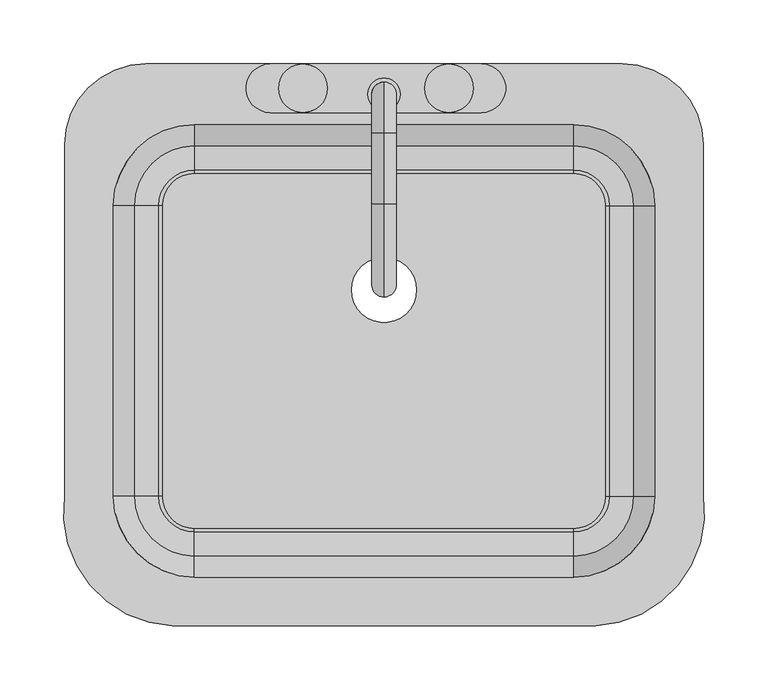
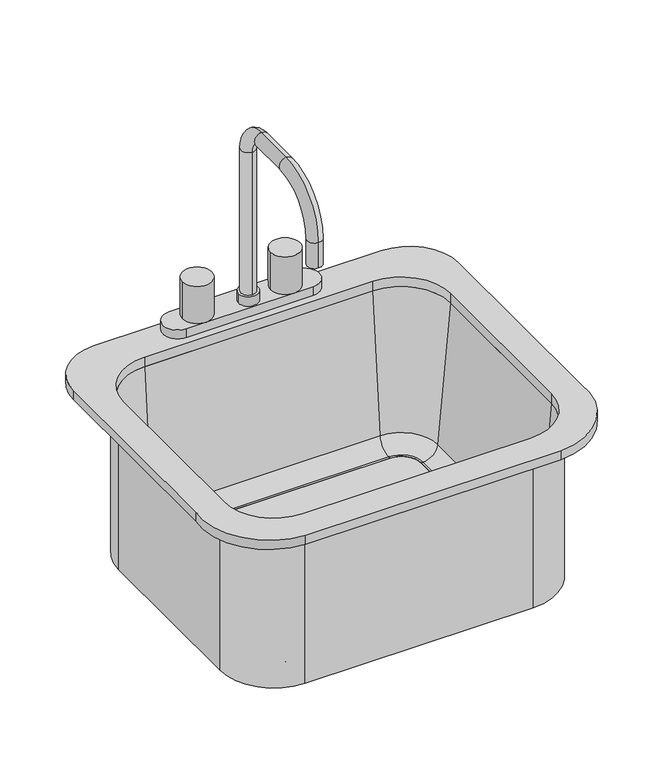
"""IFC4 building model written with IfcOpenShell, lengths in millimetres: flow terminal geometry."""

from ifc_helpers import new_model, si_unit, point, frame, frame_2d, origin, place, context, project, spatial, polyline, circle_curve, ellipse_curve, trimmed, segment, composite_curve, outline, extrude, source, transform, mapped, element, save
from ifc_brep_helpers import plane_surface, cylinder_surface, revolved_surface, advanced_brep


def flow_terminal_f629513f(model_context):
    return source(origin(), model_context, "Body", "SolidModel", [
        extrude(outline(composite_curve([segment(trimmed(circle_curve(frame_2d((-146.1534746, -170.8793432)), 89.0566732), [point((-149.9606923, -259.8545989))], [point((-234.3107593, -158.2545982))], False, "CARTESIAN"), True, "CONTINUOUS"), segment(polyline([(-234.3107593, -158.2545982), (-234.3107593, 116.6454011)]), True, "CONTINUOUS"), segment(trimmed(circle_curve(frame_2d((-170.8107593, 116.6454011)), 63.5), [point((-234.3107593, 116.6454011))], [point((-170.8107593, 180.1454011))], False, "CARTESIAN"), True, "CONTINUOUS"), segment(polyline([(-170.8107593, 180.1454011), (202.1892406, 180.1454011)]), True, "CONTINUOUS"), segment(trimmed(circle_curve(frame_2d((202.1892406, 116.6454011)), 63.5), [point((202.1892406, 180.1454011))], [point((265.6892406, 116.6454011))], False, "CARTESIAN"), True, "CONTINUOUS"), segment(polyline([(265.6892406, 116.6454011), (265.6892406, -158.2545989)]), True, "CONTINUOUS"), segment(trimmed(circle_curve(frame_2d((177.5319557, -170.8793432)), 89.0566732), [point((265.6892406, -158.2545989))], [point((181.3391735, -259.8545989))], False, "CARTESIAN"), True, "CONTINUOUS"), segment(polyline([(181.3391735, -259.8545989), (-149.9606923, -259.8545989)]), True, "CONTINUOUS")], self_intersect=False), holes=[composite_curve([segment(polyline([(164.0892406, 132.5204011), (-132.7107594, 132.5204011)]), True, "CONTINUOUS"), segment(trimmed(circle_curve(frame_2d((-132.7107594, 69.0204011)), 63.5), [point((-132.7107594, 132.5204011))], [point((-196.2107594, 69.0204011))], True, "CARTESIAN"), True, "CONTINUOUS"), segment(polyline([(-196.2107594, 69.0204011), (-196.2107594, -158.2545989)]), True, "CONTINUOUS"), segment(trimmed(circle_curve(frame_2d((-132.7107594, -158.2545989)), 63.5), [point((-196.2107594, -158.2545989))], [point((-132.7107594, -221.7545989))], True, "CARTESIAN"), True, "CONTINUOUS"), segment(polyline([(-132.7107594, -221.7545989), (164.0892406, -221.7545989)]), True, "CONTINUOUS"), segment(trimmed(circle_curve(frame_2d((164.0892406, -158.2545989)), 63.5), [point((164.0892406, -221.7545989))], [point((227.5892406, -158.2545989))], True, "CARTESIAN"), True, "CONTINUOUS"), segment(polyline([(227.5892406, -158.2545989), (227.5892406, 69.0204011)]), True, "CONTINUOUS"), segment(trimmed(circle_curve(frame_2d((164.0892406, 69.0204011)), 63.5), [point((227.5892406, 69.0204011))], [point((164.0892406, 132.5204011))], True, "CARTESIAN"), True, "CONTINUOUS")], self_intersect=False)]), frame((0.0, 0.0, 750.0), z_axis=(0.0, 0.0, 1.0), x_axis=(1.0, 0.0, 0.0)), (0.0, 0.0, 1.0), 12.7),
        advanced_brep(
        [(233.9392406, 69.0204011, 534.1), (164.0892406, 138.8704011, 534.1), (164.0892406, 138.8704011, 750.0), (233.9392406, 69.0204011, 750.0), (189.4892406, 69.0204011, 534.1), (164.0892406, 94.4204011, 534.1), (189.4892406, 69.0204011, 543.625), (164.0892406, 94.4204011, 543.625), (192.0776588, 69.0204011, 543.625), (164.0892406, 97.0088193, 543.625), (211.0551678, 69.0204011, 561.0146831), (164.0892406, 115.9863283, 561.0146831), (227.5892406, 69.0204011, 750.0), (164.0892406, 132.5204011, 750.0), (233.9392406, -158.2545989, 750.0), (233.9392406, -158.2545989, 534.1), (189.4892406, -158.2545989, 534.1), (189.4892406, -158.2545989, 543.625), (192.0776588, -158.2545989, 543.625), (211.0551678, -158.2545989, 561.0146831), (227.5892406, -158.2545989, 750.0), (164.0892406, -228.1045989, 534.1), (164.0892406, -228.1045989, 750.0), (164.0892406, -183.6545989, 534.1), (164.0892406, -183.6545989, 543.625), (164.0892406, -186.2430171, 543.625), (164.0892406, -205.2205261, 561.0146831), (164.0892406, -221.7545989, 750.0), (-132.7107594, -228.1045989, 750.0), (-132.7107594, -228.1045989, 534.1), (-132.7107594, -183.6545989, 534.1), (-132.7107594, -183.6545989, 543.625), (-132.7107594, -186.2430171, 543.625), (-132.7107594, -205.2205261, 561.0146831), (-132.7107594, -221.7545989, 750.0), (-202.5607594, -158.2545989, 534.1), (-202.5607594, -158.2545989, 750.0), (-158.1107594, -158.2545989, 534.1), (-158.1107594, -158.2545989, 543.625), (-160.6991776, -158.2545989, 543.625), (-179.6766866, -158.2545989, 561.0146831), (-196.2107594, -158.2545989, 750.0), (-202.5607594, 69.0204011, 750.0), (-202.5607594, 69.0204011, 534.1), (-158.1107594, 69.0204011, 534.1), (-158.1107594, 69.0204011, 543.625), (-160.6991776, 69.0204011, 543.625), (-179.6766866, 69.0204011, 561.0146831), (-196.2107594, 69.0204011, 750.0), (-132.7107594, 138.8704011, 534.1), (-132.7107594, 138.8704011, 750.0), (-132.7107594, 94.4204011, 534.1), (-132.7107594, 94.4204011, 543.625), (-132.7107594, 97.0088193, 543.625), (-132.7107594, 115.9863283, 561.0146831), (-132.7107594, 132.5204011, 750.0)],
        [
            (0, 1, circle_curve(frame((164.0892406, 69.0204011, 534.1), z_axis=(0.0, 0.0, 1.0), x_axis=(0.0, 1.0, 0.0)), 69.85)),
            (1, 2),
            (2, 3, circle_curve(frame((164.0892406, 69.0204011, 750.0), z_axis=(0.0, 0.0, -1.0), x_axis=(0.0, 1.0, 0.0)), 69.85)),
            (3, 0),
            (4, 5, circle_curve(frame((164.0892406, 69.0204011, 534.1), z_axis=(0.0, 0.0, 1.0), x_axis=(0.0, 1.0, 0.0)), 25.4)),
            (5, 1),
            (0, 4),
            (6, 7, circle_curve(frame((164.0892406, 69.0204011, 543.625), z_axis=(0.0, 0.0, 1.0), x_axis=(0.0, 1.0, 0.0)), 25.4)),
            (7, 5),
            (4, 6),
            (8, 9, circle_curve(frame((164.0892406, 69.0204011, 543.625), z_axis=(0.0, 0.0, 1.0), x_axis=(0.0, 1.0, 0.0)), 27.9884182)),
            (9, 7),
            (6, 8),
            (10, 11, circle_curve(frame((164.0892406, 69.0204011, 561.0146831), z_axis=(0.0, 0.0, 1.0), x_axis=(0.0, 1.0, 0.0)), 46.9659272)),
            (11, 9, circle_curve(frame((164.0892406, 97.0088193, 562.675), z_axis=(-1.0, 0.0, 0.0), x_axis=(0.0, 1.0, 0.0)), 19.05)),
            (8, 10, circle_curve(frame((192.0776588, 69.0204011, 562.675), z_axis=(0.0, -1.0, 0.0), x_axis=(1.0, 0.0, 0.0)), 19.05)),
            (12, 13, circle_curve(frame((164.0892406, 69.0204011, 750.0), z_axis=(0.0, 0.0, 1.0), x_axis=(0.0, 1.0, 0.0)), 63.5)),
            (13, 11),
            (10, 12),
            (2, 13),
            (12, 3),
            (3, 14),
            (14, 15),
            (15, 0),
            (15, 16),
            (16, 4),
            (16, 17),
            (17, 6),
            (17, 18),
            (18, 8),
            (18, 19, circle_curve(frame((192.0776588, -158.2545989, 562.675), z_axis=(0.0, -1.0, 0.0), x_axis=(1.0, 0.0, 0.0)), 19.05)),
            (19, 10),
            (19, 20),
            (20, 12),
            (20, 14),
            (21, 15, circle_curve(frame((164.0892406, -158.2545989, 534.1), z_axis=(0.0, 0.0, 1.0), x_axis=(1.0, 0.0, 0.0)), 69.85)),
            (14, 22, circle_curve(frame((164.0892406, -158.2545989, 750.0), z_axis=(0.0, 0.0, -1.0), x_axis=(1.0, 0.0, 0.0)), 69.85)),
            (22, 21),
            (23, 16, circle_curve(frame((164.0892406, -158.2545989, 534.1), z_axis=(0.0, 0.0, 1.0), x_axis=(1.0, 0.0, 0.0)), 25.4)),
            (21, 23),
            (24, 17, circle_curve(frame((164.0892406, -158.2545989, 543.625), z_axis=(0.0, 0.0, 1.0), x_axis=(1.0, 0.0, 0.0)), 25.4)),
            (23, 24),
            (25, 18, circle_curve(frame((164.0892406, -158.2545989, 543.625), z_axis=(0.0, 0.0, 1.0), x_axis=(1.0, 0.0, 0.0)), 27.9884182)),
            (24, 25),
            (26, 19, circle_curve(frame((164.0892406, -158.2545989, 561.0146831), z_axis=(0.0, 0.0, 1.0), x_axis=(1.0, 0.0, 0.0)), 46.9659272)),
            (25, 26, circle_curve(frame((164.0892406, -186.2430171, 562.675), z_axis=(-1.0, 0.0, 0.0), x_axis=(0.0, -1.0, 0.0)), 19.05)),
            (27, 20, circle_curve(frame((164.0892406, -158.2545989, 750.0), z_axis=(0.0, 0.0, 1.0), x_axis=(1.0, 0.0, 0.0)), 63.5)),
            (26, 27),
            (27, 22),
            (22, 28),
            (28, 29),
            (29, 21),
            (29, 30),
            (30, 23),
            (30, 31),
            (31, 24),
            (31, 32),
            (32, 25),
            (32, 33, circle_curve(frame((-132.7107594, -186.2430171, 562.675), z_axis=(-1.0, 0.0, 0.0), x_axis=(0.0, -1.0, 0.0)), 19.05)),
            (33, 26),
            (33, 34),
            (34, 27),
            (34, 28),
            (35, 29, circle_curve(frame((-132.7107594, -158.2545989, 534.1), z_axis=(0.0, 0.0, 1.0), x_axis=(0.0, -1.0, 0.0)), 69.85)),
            (28, 36, circle_curve(frame((-132.7107594, -158.2545989, 750.0), z_axis=(0.0, 0.0, -1.0), x_axis=(0.0, -1.0, 0.0)), 69.85)),
            (36, 35),
            (37, 30, circle_curve(frame((-132.7107594, -158.2545989, 534.1), z_axis=(0.0, 0.0, 1.0), x_axis=(0.0, -1.0, 0.0)), 25.4)),
            (35, 37),
            (38, 31, circle_curve(frame((-132.7107594, -158.2545989, 543.625), z_axis=(0.0, 0.0, 1.0), x_axis=(0.0, -1.0, 0.0)), 25.4)),
            (37, 38),
            (39, 32, circle_curve(frame((-132.7107594, -158.2545989, 543.625), z_axis=(0.0, 0.0, 1.0), x_axis=(0.0, -1.0, 0.0)), 27.9884182)),
            (38, 39),
            (40, 33, circle_curve(frame((-132.7107594, -158.2545989, 561.0146831), z_axis=(0.0, 0.0, 1.0), x_axis=(0.0, -1.0, 0.0)), 46.9659272)),
            (39, 40, circle_curve(frame((-160.6991776, -158.2545989, 562.675), z_axis=(0.0, 1.0, 0.0), x_axis=(-1.0, 0.0, 0.0)), 19.05)),
            (41, 34, circle_curve(frame((-132.7107594, -158.2545989, 750.0), z_axis=(0.0, 0.0, 1.0), x_axis=(0.0, -1.0, 0.0)), 63.5)),
            (40, 41),
            (41, 36),
            (36, 42),
            (42, 43),
            (43, 35),
            (43, 44),
            (44, 37),
            (44, 45),
            (45, 38),
            (45, 46),
            (46, 39),
            (46, 47, circle_curve(frame((-160.6991776, 69.0204011, 562.675), z_axis=(0.0, 1.0, 0.0), x_axis=(-1.0, 0.0, 0.0)), 19.05)),
            (47, 40),
            (47, 48),
            (48, 41),
            (48, 42),
            (49, 43, circle_curve(frame((-132.7107594, 69.0204011, 534.1), z_axis=(0.0, 0.0, 1.0), x_axis=(-1.0, 0.0, 0.0)), 69.85)),
            (42, 50, circle_curve(frame((-132.7107594, 69.0204011, 750.0), z_axis=(0.0, 0.0, -1.0), x_axis=(-1.0, 0.0, 0.0)), 69.85)),
            (50, 49),
            (51, 44, circle_curve(frame((-132.7107594, 69.0204011, 534.1), z_axis=(0.0, 0.0, 1.0), x_axis=(-1.0, 0.0, 0.0)), 25.4)),
            (49, 51),
            (52, 45, circle_curve(frame((-132.7107594, 69.0204011, 543.625), z_axis=(0.0, 0.0, 1.0), x_axis=(-1.0, 0.0, 0.0)), 25.4)),
            (51, 52),
            (53, 46, circle_curve(frame((-132.7107594, 69.0204011, 543.625), z_axis=(0.0, 0.0, 1.0), x_axis=(-1.0, 0.0, 0.0)), 27.9884182)),
            (52, 53),
            (54, 47, circle_curve(frame((-132.7107594, 69.0204011, 561.0146831), z_axis=(0.0, 0.0, 1.0), x_axis=(-1.0, 0.0, 0.0)), 46.9659272)),
            (53, 54, circle_curve(frame((-132.7107594, 97.0088193, 562.675), z_axis=(1.0, 0.0, 0.0), x_axis=(0.0, 1.0, 0.0)), 19.05)),
            (55, 48, circle_curve(frame((-132.7107594, 69.0204011, 750.0), z_axis=(0.0, 0.0, 1.0), x_axis=(-1.0, 0.0, 0.0)), 63.5)),
            (54, 55),
            (55, 50),
            (50, 2),
            (1, 49),
            (5, 51),
            (7, 52),
            (9, 53),
            (11, 54),
            (13, 55),
        ],
        [
            cylinder_surface(frame((164.0892406, 69.0204011, 0.0), z_axis=(0.0, 0.0, -1.0), x_axis=(0.0, 1.0, 0.0)), 69.85),
            plane_surface(frame((164.0892406, 69.0204011, 534.1), z_axis=(0.0, 0.0, -1.0), x_axis=(0.0, 1.0, 0.0))),
            revolved_surface(polyline([(164.0892406, 94.42040109999999, 534.1), (164.0892406, 94.42040109999999, 543.625)]), (164.0892406, 69.0204011, 0.0), (0.0, 0.0, -1.0)),
            plane_surface(frame((164.0892406, 69.0204011, 543.625), z_axis=(0.0, 0.0, 1.0), x_axis=(0.0, 1.0, 0.0))),
            revolved_surface(trimmed(ellipse_curve(frame((164.0892406, 97.0088193, 562.675), z_axis=(1.0, 0.0, 0.0), x_axis=(0.0, 1.0, 0.0)), 19.05, 19.05), [point((164.0892406, 97.0088193, 543.625))], [point((164.0892406, 115.9863283, 561.0146831))], True, "CARTESIAN"), (164.0892406, 69.0204011, 0.0), (0.0, 0.0, -1.0)),
            revolved_surface(polyline([(164.0892406, 115.9863283, 561.0146831), (164.0892406, 132.5204011, 750.0)]), (164.0892406, 69.0204011, 0.0), (0.0, 0.0, -1.0)),
            plane_surface(frame((164.0892406, 69.0204011, 750.0), z_axis=(0.0, 0.0, 1.0), x_axis=(0.0, 1.0, 0.0))),
            plane_surface(frame((233.9392406, 69.0204011, 750.0), z_axis=(1.0, 0.0, 0.0), x_axis=(0.0, -1.0, 0.0))),
            plane_surface(frame((233.9392406, 69.0204011, 534.1), z_axis=(0.0, 0.0, -1.0), x_axis=(0.0, -1.0, 0.0))),
            plane_surface(frame((189.4892406, 69.0204011, 534.1), z_axis=(-1.0, 0.0, 0.0), x_axis=(0.0, -1.0, 0.0))),
            plane_surface(frame((189.4892406, 69.0204011, 543.625), z_axis=(0.0, 0.0, 1.0), x_axis=(0.0, -1.0, 0.0))),
            revolved_surface(polyline([(211.1276588, -158.25459889999996, 562.675), (211.1276588, 69.0204011, 562.675)]), (192.0776588, 69.0204011, 562.675), (0.0, -1.0, 0.0)),
            plane_surface(frame((211.0551678, 69.0204011, 561.0146831), z_axis=(-0.9961946980917442, 0.0, 0.0871557427476735), x_axis=(0.0, -1.0, 0.0))),
            plane_surface(frame((227.5892406, 69.0204011, 750.0), z_axis=(0.0, 0.0, 1.0), x_axis=(0.0, -1.0, 0.0))),
            cylinder_surface(frame((164.0892406, -158.2545989, 0.0), z_axis=(0.0, 0.0, -1.0), x_axis=(1.0, 0.0, 0.0)), 69.85),
            plane_surface(frame((164.0892406, -158.2545989, 534.1), z_axis=(0.0, 0.0, -1.0), x_axis=(1.0, 0.0, 0.0))),
            revolved_surface(polyline([(189.48924060000002, -158.2545989, 534.1), (189.48924060000002, -158.2545989, 543.625)]), (164.0892406, -158.2545989, 0.0), (0.0, 0.0, -1.0)),
            plane_surface(frame((164.0892406, -158.2545989, 543.625), z_axis=(0.0, 0.0, 1.0), x_axis=(1.0, 0.0, 0.0))),
            revolved_surface(trimmed(ellipse_curve(frame((192.0776588, -158.2545989, 562.675), z_axis=(0.0, -1.0, 0.0), x_axis=(1.0, 0.0, 0.0)), 19.05, 19.05), [point((192.0776588, -158.2545989, 543.625))], [point((211.0551678, -158.2545989, 561.0146831))], True, "CARTESIAN"), (164.0892406, -158.2545989, 0.0), (0.0, 0.0, -1.0)),
            revolved_surface(polyline([(211.0551678, -158.2545989, 561.0146831), (227.5892406, -158.2545989, 750.0)]), (164.0892406, -158.2545989, 0.0), (0.0, 0.0, -1.0)),
            plane_surface(frame((164.0892406, -158.2545989, 750.0), z_axis=(0.0, 0.0, 1.0), x_axis=(1.0, 0.0, 0.0))),
            plane_surface(frame((164.0892406, -228.1045989, 750.0), z_axis=(0.0, -1.0, 0.0), x_axis=(-1.0, 0.0, 0.0))),
            plane_surface(frame((164.0892406, -228.1045989, 534.1), z_axis=(0.0, 0.0, -1.0), x_axis=(-1.0, 0.0, 0.0))),
            plane_surface(frame((164.0892406, -183.6545989, 534.1), z_axis=(0.0, 1.0, 0.0), x_axis=(-1.0, 0.0, 0.0))),
            plane_surface(frame((164.0892406, -183.6545989, 543.625), z_axis=(0.0, 0.0, 1.0), x_axis=(-1.0, 0.0, 0.0))),
            revolved_surface(polyline([(-132.7107594, -205.29301710000001, 562.675), (164.0892406, -205.29301710000001, 562.675)]), (164.0892406, -186.2430171, 562.675), (-1.0, 0.0, 0.0)),
            plane_surface(frame((164.0892406, -205.2205261, 561.0146831), z_axis=(0.0, 0.9961946980917442, 0.0871557427476735), x_axis=(-1.0, 0.0, 0.0))),
            plane_surface(frame((164.0892406, -221.7545989, 750.0), z_axis=(0.0, 0.0, 1.0), x_axis=(-1.0, 0.0, 0.0))),
            cylinder_surface(frame((-132.7107594, -158.2545989, 0.0), z_axis=(0.0, 0.0, -1.0), x_axis=(0.0, -1.0, 0.0)), 69.85),
            plane_surface(frame((-132.7107594, -158.2545989, 534.1), z_axis=(0.0, 0.0, -1.0), x_axis=(0.0, -1.0, 0.0))),
            revolved_surface(polyline([(-132.7107594, -183.6545989, 534.1), (-132.7107594, -183.6545989, 543.625)]), (-132.7107594, -158.2545989, 0.0), (0.0, 0.0, -1.0)),
            plane_surface(frame((-132.7107594, -158.2545989, 543.625), z_axis=(0.0, 0.0, 1.0), x_axis=(0.0, -1.0, 0.0))),
            revolved_surface(trimmed(ellipse_curve(frame((-132.7107594, -186.2430171, 562.675), z_axis=(-1.0, 0.0, 0.0), x_axis=(0.0, -1.0, 0.0)), 19.05, 19.05), [point((-132.7107594, -186.2430171, 543.625))], [point((-132.7107594, -205.2205261, 561.0146831))], True, "CARTESIAN"), (-132.7107594, -158.2545989, 0.0), (0.0, 0.0, -1.0)),
            revolved_surface(polyline([(-132.7107594, -205.2205261, 561.0146831), (-132.7107594, -221.7545989, 750.0)]), (-132.7107594, -158.2545989, 0.0), (0.0, 0.0, -1.0)),
            plane_surface(frame((-132.7107594, -158.2545989, 750.0), z_axis=(0.0, 0.0, 1.0), x_axis=(0.0, -1.0, 0.0))),
            plane_surface(frame((-202.5607594, -158.2545989, 750.0), z_axis=(-1.0, 0.0, 0.0), x_axis=(0.0, 1.0, 0.0))),
            plane_surface(frame((-202.5607594, -158.2545989, 534.1), z_axis=(0.0, 0.0, -1.0), x_axis=(0.0, 1.0, 0.0))),
            plane_surface(frame((-158.1107594, -158.2545989, 534.1), z_axis=(1.0, 0.0, 0.0), x_axis=(0.0, 1.0, 0.0))),
            plane_surface(frame((-158.1107594, -158.2545989, 543.625), z_axis=(0.0, 0.0, 1.0), x_axis=(0.0, 1.0, 0.0))),
            revolved_surface(polyline([(-179.74917760000002, 69.02040109999999, 562.675), (-179.74917760000002, -158.2545989, 562.675)]), (-160.6991776, -158.2545989, 562.675), (0.0, 1.0, 0.0)),
            plane_surface(frame((-179.6766866, -158.2545989, 561.0146831), z_axis=(0.9961946980917442, 0.0, 0.0871557427476735), x_axis=(0.0, 1.0, 0.0))),
            plane_surface(frame((-196.2107594, -158.2545989, 750.0), z_axis=(0.0, 0.0, 1.0), x_axis=(0.0, 1.0, 0.0))),
            cylinder_surface(frame((-132.7107594, 69.0204011, 0.0), z_axis=(0.0, 0.0, -1.0), x_axis=(-1.0, 0.0, 0.0)), 69.85),
            plane_surface(frame((-132.7107594, 69.0204011, 534.1), z_axis=(0.0, 0.0, -1.0), x_axis=(-1.0, 0.0, 0.0))),
            revolved_surface(polyline([(-158.1107594, 69.0204011, 534.1), (-158.1107594, 69.0204011, 543.625)]), (-132.7107594, 69.0204011, 0.0), (0.0, 0.0, -1.0)),
            plane_surface(frame((-132.7107594, 69.0204011, 543.625), z_axis=(0.0, 0.0, 1.0), x_axis=(-1.0, 0.0, 0.0))),
            revolved_surface(trimmed(ellipse_curve(frame((-160.6991776, 69.0204011, 562.675), z_axis=(0.0, 1.0, 0.0), x_axis=(-1.0, 0.0, 0.0)), 19.05, 19.05), [point((-160.6991776, 69.0204011, 543.625))], [point((-179.6766866, 69.0204011, 561.0146831))], True, "CARTESIAN"), (-132.7107594, 69.0204011, 0.0), (0.0, 0.0, -1.0)),
            revolved_surface(polyline([(-179.6766866, 69.0204011, 561.0146831), (-196.2107594, 69.0204011, 750.0)]), (-132.7107594, 69.0204011, 0.0), (0.0, 0.0, -1.0)),
            plane_surface(frame((-132.7107594, 69.0204011, 750.0), z_axis=(0.0, 0.0, 1.0), x_axis=(-1.0, 0.0, 0.0))),
            plane_surface(frame((-132.7107594, 138.8704011, 750.0), z_axis=(0.0, 1.0, 0.0), x_axis=(1.0, 0.0, 0.0))),
            plane_surface(frame((-132.7107594, 138.8704011, 534.1), z_axis=(0.0, 0.0, -1.0), x_axis=(1.0, 0.0, 0.0))),
            plane_surface(frame((-132.7107594, 94.4204011, 534.1), z_axis=(0.0, -1.0, 0.0), x_axis=(1.0, 0.0, 0.0))),
            plane_surface(frame((-132.7107594, 94.4204011, 543.625), z_axis=(0.0, 0.0, 1.0), x_axis=(1.0, 0.0, 0.0))),
            revolved_surface(polyline([(164.0892406, 116.0588193, 562.675), (-132.7107594, 116.0588193, 562.675)]), (-132.7107594, 97.0088193, 562.675), (1.0, 0.0, 0.0)),
            plane_surface(frame((-132.7107594, 115.9863283, 561.0146831), z_axis=(0.0, -0.9961946980917442, 0.0871557427476735), x_axis=(1.0, 0.0, 0.0))),
            plane_surface(frame((-132.7107594, 132.5204011, 750.0), z_axis=(0.0, 0.0, 1.0), x_axis=(1.0, 0.0, 0.0))),
        ],
        [
            (0, [[1, 2, 3, 4]]),
            (1, [[5, 6, -1, 7]]),
            (2, [[8, 9, -5, 10]]),
            (3, [[11, 12, -8, 13]]),
            (4, [[14, 15, -11, 16]]),
            (5, [[17, 18, -14, 19]]),
            (6, [[-3, 20, -17, 21]]),
            (7, [[-4, 22, 23, 24]]),
            (8, [[-7, -24, 25, 26]]),
            (9, [[-10, -26, 27, 28]]),
            (10, [[-13, -28, 29, 30]]),
            (11, [[-16, -30, 31, 32]]),
            (12, [[-19, -32, 33, 34]]),
            (13, [[-21, -34, 35, -22]]),
            (14, [[36, -23, 37, 38]]),
            (15, [[39, -25, -36, 40]]),
            (16, [[41, -27, -39, 42]]),
            (17, [[43, -29, -41, 44]]),
            (18, [[45, -31, -43, 46]]),
            (19, [[47, -33, -45, 48]]),
            (20, [[-37, -35, -47, 49]]),
            (21, [[-38, 50, 51, 52]]),
            (22, [[-40, -52, 53, 54]]),
            (23, [[-42, -54, 55, 56]]),
            (24, [[-44, -56, 57, 58]]),
            (25, [[-46, -58, 59, 60]]),
            (26, [[-48, -60, 61, 62]]),
            (27, [[-49, -62, 63, -50]]),
            (28, [[64, -51, 65, 66]]),
            (29, [[67, -53, -64, 68]]),
            (30, [[69, -55, -67, 70]]),
            (31, [[71, -57, -69, 72]]),
            (32, [[73, -59, -71, 74]]),
            (33, [[75, -61, -73, 76]]),
            (34, [[-65, -63, -75, 77]]),
            (35, [[-66, 78, 79, 80]]),
            (36, [[-68, -80, 81, 82]]),
            (37, [[-70, -82, 83, 84]]),
            (38, [[-72, -84, 85, 86]]),
            (39, [[-74, -86, 87, 88]]),
            (40, [[-76, -88, 89, 90]]),
            (41, [[-77, -90, 91, -78]]),
            (42, [[92, -79, 93, 94]]),
            (43, [[95, -81, -92, 96]]),
            (44, [[97, -83, -95, 98]]),
            (45, [[99, -85, -97, 100]]),
            (46, [[101, -87, -99, 102]]),
            (47, [[103, -89, -101, 104]]),
            (48, [[-93, -91, -103, 105]]),
            (49, [[-94, 106, -2, 107]]),
            (50, [[-96, -107, -6, 108]]),
            (51, [[-98, -108, -9, 109]]),
            (52, [[-100, -109, -12, 110]]),
            (53, [[-102, -110, -15, 111]]),
            (54, [[-104, -111, -18, 112]]),
            (55, [[-105, -112, -20, -106]]),
        ],
    ),
        extrude(outline(composite_curve([segment(trimmed(circle_curve(frame_2d((164.0892406, 69.0204011)), 25.4), [point((164.0892406, 94.4204011))], [point((189.4892406, 69.0204011))], False, "CARTESIAN"), True, "CONTINUOUS"), segment(polyline([(189.4892406, 69.0204011), (189.4892406, -158.2545989)]), True, "CONTINUOUS"), segment(trimmed(circle_curve(frame_2d((164.0892406, -158.2545989)), 25.4), [point((189.4892406, -158.2545989))], [point((164.0892406, -183.6545989))], False, "CARTESIAN"), True, "CONTINUOUS"), segment(polyline([(164.0892406, -183.6545989), (-132.7107594, -183.6545989)]), True, "CONTINUOUS"), segment(trimmed(circle_curve(frame_2d((-132.7107594, -158.2545989)), 25.4), [point((-132.7107594, -183.6545989))], [point((-158.1107594, -158.2545989))], False, "CARTESIAN"), True, "CONTINUOUS"), segment(polyline([(-158.1107594, -158.2545989), (-158.1107594, 69.0204011)]), True, "CONTINUOUS"), segment(trimmed(circle_curve(frame_2d((-132.7107594, 69.0204011)), 25.4), [point((-158.1107594, 69.0204011))], [point((-132.7107594, 94.4204011))], False, "CARTESIAN"), True, "CONTINUOUS"), segment(polyline([(-132.7107594, 94.4204011), (164.0892406, 94.4204011)]), True, "CONTINUOUS")], self_intersect=False), holes=[composite_curve([segment(trimmed(circle_curve(frame_2d((15.6892406, 3.175)), 25.4), [point((-9.7107594, 3.175))], [point((41.0892406, 3.175))], True, "CARTESIAN"), True, "CONTINUOUS"), segment(trimmed(circle_curve(frame_2d((15.6892406, 3.175)), 25.4), [point((41.0892406, 3.175))], [point((-9.7107594, 3.175))], True, "CARTESIAN"), True, "CONTINUOUS")], self_intersect=False)]), frame((0.0, 0.0, 534.1), z_axis=(0.0, 0.0, 1.0), x_axis=(1.0, 0.0, 0.0)), (0.0, 0.0, 1.0), 9.525),
        advanced_brep(
        [(-66.8607594, 161.0954011, 826.2), (-28.7607594, 161.0954011, 826.2), (47.4392406, 161.0954011, 826.2), (85.5392406, 161.0954011, 826.2), (91.8892406, 180.1454011, 762.7), (91.8892406, 142.0454011, 762.7), (-73.2107594, 142.0454011, 762.7), (-73.2107594, 180.1454011, 762.7), (-66.8607594, 161.0954011, 775.2), (-47.8107594, 142.0454011, 775.2), (-28.7607594, 161.0954011, 775.2), (-47.8107594, 180.1454011, 775.2), (47.4392406, 161.0954011, 775.2), (66.4892406, 142.0454011, 775.2), (85.5392406, 161.0954011, 775.2), (66.4892406, 180.1454011, 775.2), (-73.2107594, 180.1454011, 775.2), (-73.2107594, 142.0454011, 775.2), (91.8892406, 142.0454011, 775.2), (91.8892406, 180.1454011, 775.2), (28.3892406, 156.3329011, 775.2), (2.9892406, 156.3329011, 775.2), (15.6892406, 165.8579011, 983.3625), (15.6892406, 146.8079011, 983.3625), (15.6892406, 146.8079011, 788.1), (15.6892406, 165.8579011, 788.1), (15.6892406, 126.1704011, 1023.05), (15.6892406, 126.1704011, 1004.0), (15.6892406, 70.6079011, 1023.05), (15.6892406, 70.6079011, 1004.0), (15.6892406, -2.4170989, 950.025), (15.6892406, 16.6329011, 950.025), (15.6892406, -2.4170989, 915.1), (15.6892406, 16.6329011, 915.1), (2.9892406, 156.3329011, 788.1), (28.3892406, 156.3329011, 788.1)],
        [
            (0, 1, circle_curve(frame((-47.8107594, 161.0954011, 826.2), z_axis=(0.0, 0.0, 1.0), x_axis=(1.0, 0.0, 0.0)), 19.05)),
            (1, 0, circle_curve(frame((-47.8107594, 161.0954011, 826.2), z_axis=(0.0, 0.0, 1.0), x_axis=(1.0, 0.0, 0.0)), 19.05)),
            (2, 3, circle_curve(frame((66.4892406, 161.0954011, 826.2), z_axis=(0.0, 0.0, 1.0), x_axis=(1.0, 0.0, 0.0)), 19.05)),
            (3, 2, circle_curve(frame((66.4892406, 161.0954011, 826.2), z_axis=(0.0, 0.0, 1.0), x_axis=(1.0, 0.0, 0.0)), 19.05)),
            (4, 5, circle_curve(frame((91.8892406, 161.0954011, 762.7), z_axis=(0.0, 0.0, -1.0), x_axis=(1.0, 0.0, 0.0)), 19.05)),
            (5, 6),
            (6, 7, circle_curve(frame((-73.2107594, 161.0954011, 762.7), z_axis=(0.0, 0.0, -1.0), x_axis=(1.0, 0.0, 0.0)), 19.05)),
            (7, 4),
            (0, 8),
            (8, 9, circle_curve(frame((-47.8107594, 161.0954011, 775.2), z_axis=(0.0, 0.0, 1.0), x_axis=(1.0, 0.0, 0.0)), 19.05)),
            (9, 10, circle_curve(frame((-47.8107594, 161.0954011, 775.2), z_axis=(0.0, 0.0, 1.0), x_axis=(1.0, 0.0, 0.0)), 19.05)),
            (10, 1),
            (10, 11, circle_curve(frame((-47.8107594, 161.0954011, 775.2), z_axis=(0.0, 0.0, 1.0), x_axis=(1.0, 0.0, 0.0)), 19.05)),
            (11, 8, circle_curve(frame((-47.8107594, 161.0954011, 775.2), z_axis=(0.0, 0.0, 1.0), x_axis=(1.0, 0.0, 0.0)), 19.05)),
            (2, 12),
            (12, 13, circle_curve(frame((66.4892406, 161.0954011, 775.2), z_axis=(0.0, 0.0, 1.0), x_axis=(1.0, 0.0, 0.0)), 19.05)),
            (13, 14, circle_curve(frame((66.4892406, 161.0954011, 775.2), z_axis=(0.0, 0.0, 1.0), x_axis=(1.0, 0.0, 0.0)), 19.05)),
            (14, 3),
            (14, 15, circle_curve(frame((66.4892406, 161.0954011, 775.2), z_axis=(0.0, 0.0, 1.0), x_axis=(1.0, 0.0, 0.0)), 19.05)),
            (15, 12, circle_curve(frame((66.4892406, 161.0954011, 775.2), z_axis=(0.0, 0.0, 1.0), x_axis=(1.0, 0.0, 0.0)), 19.05)),
            (16, 17, circle_curve(frame((-73.2107594, 161.0954011, 775.2), z_axis=(0.0, 0.0, 1.0), x_axis=(1.0, 0.0, 0.0)), 19.05)),
            (17, 9),
            (11, 16),
            (18, 19, circle_curve(frame((91.8892406, 161.0954011, 775.2), z_axis=(0.0, 0.0, 1.0), x_axis=(1.0, 0.0, 0.0)), 19.05)),
            (19, 15),
            (13, 18),
            (15, 11),
            (9, 13),
            (20, 21, circle_curve(frame((15.6892406, 156.3329011, 775.2), z_axis=(0.0, 0.0, -1.0), x_axis=(1.0, 0.0, 0.0)), 12.7)),
            (21, 20, circle_curve(frame((15.6892406, 156.3329011, 775.2), z_axis=(0.0, 0.0, -1.0), x_axis=(1.0, 0.0, 0.0)), 12.7)),
            (19, 4),
            (7, 16),
            (6, 17),
            (5, 18),
            (22, 23, circle_curve(frame((15.6892406, 156.3329011, 983.3625), z_axis=(0.0, 0.0, -1.0), x_axis=(0.0, -1.0, 0.0)), 9.525)),
            (23, 24),
            (24, 25, circle_curve(frame((15.6892406, 156.3329011, 788.1), z_axis=(0.0, 0.0, 1.0), x_axis=(0.0, -1.0, 0.0)), 9.525)),
            (25, 22),
            (23, 22, circle_curve(frame((15.6892406, 156.3329011, 983.3625), z_axis=(0.0, 0.0, -1.0), x_axis=(0.0, -1.0, 0.0)), 9.525)),
            (25, 24, circle_curve(frame((15.6892406, 156.3329011, 788.1), z_axis=(0.0, 0.0, 1.0), x_axis=(0.0, -1.0, 0.0)), 9.525)),
            (22, 26, circle_curve(frame((15.6892406, 126.1704011, 983.3625), z_axis=(1.0, 0.0, 0.0), x_axis=(0.0, 1.0, 0.0)), 39.6875)),
            (26, 27, circle_curve(frame((15.6892406, 126.1704011, 1013.525), z_axis=(0.0, 1.0, 0.0), x_axis=(0.0, 0.0, -1.0)), 9.525)),
            (27, 23, circle_curve(frame((15.6892406, 126.1704011, 983.3625), z_axis=(-1.0, 0.0, 0.0), x_axis=(0.0, 1.0, 0.0)), 20.6375)),
            (27, 26, circle_curve(frame((15.6892406, 126.1704011, 1013.525), z_axis=(0.0, 1.0, 0.0), x_axis=(0.0, 0.0, -1.0)), 9.525)),
            (26, 28),
            (28, 29, circle_curve(frame((15.6892406, 70.6079011, 1013.525), z_axis=(0.0, 1.0, 0.0), x_axis=(0.0, 0.0, -1.0)), 9.525)),
            (29, 27),
            (29, 28, circle_curve(frame((15.6892406, 70.6079011, 1013.525), z_axis=(0.0, 1.0, 0.0), x_axis=(0.0, 0.0, -1.0)), 9.525)),
            (28, 30, circle_curve(frame((15.6892406, 70.6079011, 950.025), z_axis=(1.0, 0.0, 0.0), x_axis=(0.0, 0.0, 1.0)), 73.025)),
            (30, 31, circle_curve(frame((15.6892406, 7.1079011, 950.025), z_axis=(0.0, 0.0, 1.0), x_axis=(0.0, 1.0, 0.0)), 9.525)),
            (31, 29, circle_curve(frame((15.6892406, 70.6079011, 950.025), z_axis=(-1.0, 0.0, 0.0), x_axis=(0.0, 0.0, 1.0)), 53.975)),
            (31, 30, circle_curve(frame((15.6892406, 7.1079011, 950.025), z_axis=(0.0, 0.0, 1.0), x_axis=(0.0, 1.0, 0.0)), 9.525)),
            (32, 33, circle_curve(frame((15.6892406, 7.1079011, 915.1), z_axis=(0.0, 0.0, -1.0), x_axis=(0.0, 1.0, 0.0)), 9.525)),
            (33, 32, circle_curve(frame((15.6892406, 7.1079011, 915.1), z_axis=(0.0, 0.0, -1.0), x_axis=(0.0, 1.0, 0.0)), 9.525)),
            (30, 32),
            (33, 31),
            (34, 35, circle_curve(frame((15.6892406, 156.3329011, 788.1), z_axis=(0.0, 0.0, 1.0), x_axis=(1.0, 0.0, 0.0)), 12.7)),
            (35, 34, circle_curve(frame((15.6892406, 156.3329011, 788.1), z_axis=(0.0, 0.0, 1.0), x_axis=(1.0, 0.0, 0.0)), 12.7)),
            (34, 21),
            (20, 35),
        ],
        [
            plane_surface(frame((-28.7607594, 161.0954011, 826.2), z_axis=(0.0, 0.0, 1.0), x_axis=(0.0, 1.0, 0.0))),
            plane_surface(frame((-28.7607594, 161.0954011, 762.7), z_axis=(0.0, 0.0, -1.0), x_axis=(0.0, -1.0, 0.0))),
            cylinder_surface(frame((-47.8107594, 161.0954011, 762.7), z_axis=(0.0, 0.0, 1.0), x_axis=(1.0, 0.0, 0.0)), 19.05),
            cylinder_surface(frame((66.4892406, 161.0954011, 0.0), z_axis=(0.0, 0.0, 1.0), x_axis=(1.0, 0.0, 0.0)), 19.05),
            plane_surface(frame((-73.2107594, 180.1454011, 775.2), z_axis=(0.0, 0.0, 1.0), x_axis=(-1.0, 0.0, 0.0))),
            plane_surface(frame((91.8892406, 180.1454011, 775.2), z_axis=(0.0, 1.0, 0.0), x_axis=(0.0, 0.0, -1.0))),
            cylinder_surface(frame((-73.2107594, 161.0954011, 762.7), z_axis=(0.0, 0.0, 1.0), x_axis=(1.0, 0.0, 0.0)), 19.05),
            plane_surface(frame((-73.2107594, 142.0454011, 775.2), z_axis=(0.0, -1.0, 0.0), x_axis=(0.0, 0.0, -1.0))),
            cylinder_surface(frame((91.8892406, 161.0954011, 762.7), z_axis=(0.0, 0.0, 1.0), x_axis=(1.0, 0.0, 0.0)), 19.05),
            cylinder_surface(frame((15.6892406, 156.3329011, 762.7), z_axis=(0.0, 0.0, -1.0), x_axis=(0.0, -1.0, 0.0)), 9.525),
            revolved_surface(trimmed(ellipse_curve(frame((15.6892406, 156.3329011, 983.3625), z_axis=(0.0, 0.0, -1.0), x_axis=(0.0, -1.0, 0.0)), 9.525, 9.525), [point((15.6892406, 165.8579011, 983.3625))], [point((15.6892406, 146.8079011, 983.3625))], True, "CARTESIAN"), (15.6892406, 126.1704011, 983.3625), (1.0, 0.0, 0.0)),
            revolved_surface(trimmed(ellipse_curve(frame((15.6892406, 156.3329011, 983.3625), z_axis=(0.0, 0.0, -1.0), x_axis=(0.0, -1.0, 0.0)), 9.525, 9.525), [point((15.6892406, 146.8079011, 983.3625))], [point((15.6892406, 165.8579011, 983.3625))], True, "CARTESIAN"), (15.6892406, 126.1704011, 983.3625), (1.0, 0.0, 0.0)),
            cylinder_surface(frame((15.6892406, 126.1704011, 1013.525), z_axis=(0.0, 1.0, 0.0), x_axis=(0.0, 0.0, -1.0)), 9.525),
            revolved_surface(trimmed(ellipse_curve(frame((15.6892406, 70.6079011, 1013.525), z_axis=(0.0, 1.0, 0.0), x_axis=(0.0, 0.0, -1.0)), 9.525, 9.525), [point((15.6892406, 70.6079011, 1023.05))], [point((15.6892406, 70.6079011, 1004.0))], True, "CARTESIAN"), (15.6892406, 70.6079011, 950.025), (1.0, 0.0, 0.0)),
            revolved_surface(trimmed(ellipse_curve(frame((15.6892406, 70.6079011, 1013.525), z_axis=(0.0, 1.0, 0.0), x_axis=(0.0, 0.0, -1.0)), 9.525, 9.525), [point((15.6892406, 70.6079011, 1004.0))], [point((15.6892406, 70.6079011, 1023.05))], True, "CARTESIAN"), (15.6892406, 70.6079011, 950.025), (1.0, 0.0, 0.0)),
            plane_surface(frame((15.6892406, -2.4170989, 915.1), z_axis=(0.0, 0.0, -1.0), x_axis=(-1.0, 0.0, 0.0))),
            cylinder_surface(frame((15.6892406, 7.1079011, 950.025), z_axis=(0.0, 0.0, 1.0), x_axis=(0.0, 1.0, 0.0)), 9.525),
            plane_surface(frame((28.3892406, 156.3329011, 788.1), z_axis=(0.0, 0.0, 1.0), x_axis=(0.0, 1.0, 0.0))),
            cylinder_surface(frame((15.6892406, 156.3329011, 762.7), z_axis=(0.0, 0.0, 1.0), x_axis=(1.0, 0.0, 0.0)), 12.7),
        ],
        [
            (0, [[1, 2]]),
            (0, [[3, 4]]),
            (1, [[5, 6, 7, 8]]),
            (2, [[-1, 9, 10, 11, 12]]),
            (2, [[-2, -12, 13, 14, -9]]),
            (3, [[-3, 15, 16, 17, 18]]),
            (3, [[-4, -18, 19, 20, -15]]),
            (4, [[21, 22, -10, -14, 23]]),
            (4, [[24, 25, -19, -17, 26]]),
            (4, [[27, -13, -11, 28, -16, -20], [29, 30]]),
            (5, [[31, -8, 32, -23, -27, -25]]),
            (6, [[-21, -32, -7, 33]]),
            (7, [[-33, -6, 34, -26, -28, -22]]),
            (8, [[-24, -34, -5, -31]]),
            (9, [[35, 36, 37, 38]]),
            (9, [[39, -38, 40, -36]]),
            (10, [[-35, 41, 42, 43]]),
            (11, [[-39, -43, 44, -41]]),
            (12, [[-42, 45, 46, 47]]),
            (12, [[-44, -47, 48, -45]]),
            (13, [[-46, 49, 50, 51]]),
            (14, [[-48, -51, 52, -49]]),
            (15, [[53, 54]]),
            (16, [[-50, 55, -54, 56]]),
            (16, [[-52, -56, -53, -55]]),
            (17, [[57, 58], [-37, -40]]),
            (18, [[-57, 59, -29, 60]]),
            (18, [[-58, -60, -30, -59]]),
        ],
    ),
    ])


if __name__ == "__main__":
    model = new_model("IFC4")
    model_context = context("Model", 3, world=origin())
    ifc_project = project(units=[si_unit("LENGTHUNIT", "METRE", prefix="MILLI")], contexts=[model_context])
    site = spatial("IfcSite", under=ifc_project)
    building = spatial("IfcBuilding", under=site)
    placement = place(None, origin())
    flow_terminal_shape = flow_terminal_f629513f(model_context)
    element("IfcFlowTerminal", 1, at=placement, inside=building, context=model_context, shape_type="MappedRepresentation", body=[
        mapped(flow_terminal_shape, transform((0.0, 0.0, 0.0), x_axis=(1.0, 0.0, 0.0), y_axis=(0.0, 1.0, 0.0), z_axis=(0.0, 0.0, 1.0))),
    ])
    save(model, "model.ifc")

# Revit data of these elements
# Type
#   Hauteur du plan de travail = 750 mm
#   Profondeur = 440 mm
#   Largeur = 500 mm
#   Default Elevation = 0
